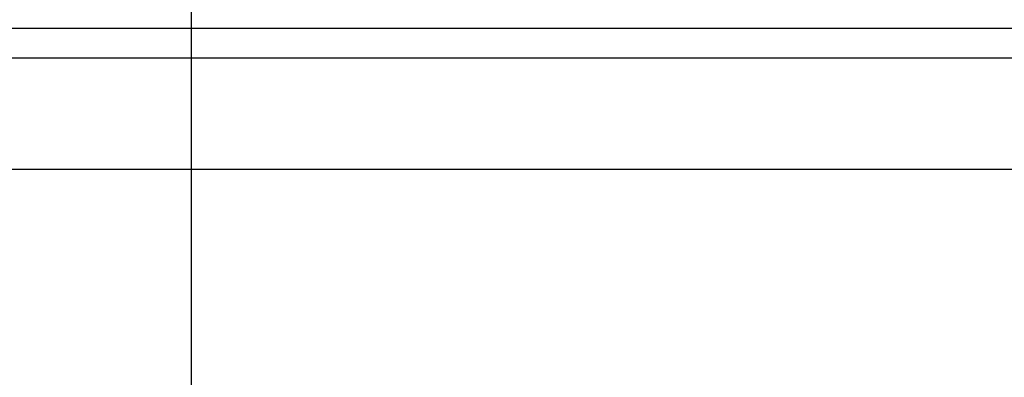
# Model space of a CAD drawing. Units: inches. Extents: x 2278 to 7495, y -71 to 1198.
# Tile 18 of 44: x 5007 to 5060, y 107 to 126. Entities that reach past the tile are written whole.
import ezdxf

# ---------------------------------------------------------------- set-up
doc = ezdxf.new("R2010")
doc.units = ezdxf.units.IN
doc.header["$MEASUREMENT"] = 0
doc.layers.add('A-ANNO-DIMS', color=2, linetype='Continuous', lineweight=18)
doc.layers.add('A-ELEV', color=7, linetype='Continuous', lineweight=25)
doc.styles.get("Standard").update_dxf_attribs({"font": 'arial.ttf'})
doc.dimstyles.get("Standard").update_dxf_attribs({"dimtxt": 6, "dimasz": 3, "dimexe": 0.18, "dimexo": 0.0625, "dimgap": 0.09, "dimtad": 0, "dimtih": 1, "dimtoh": 1, "dimdec": 0, "dimzin": 0, "dimdsep": 46, "dimlunit": 3, "dimtxsty": 'Standard', "dimblk": 'ARCHTICK', "dimcen": 0.09, "dimadec": 0, "dimazin": 0, "dimtfac": 1, "dimtdec": 0, "dimtofl": 0, "dimtmove": 0, "dimatfit": 3, "dimfxl": 1, "dimtolj": 1, "dimtzin": 0, "dimarcsym": 0})

# ---------------------------------------------------------------- blocks, each defined once
blk = doc.blocks.new('_ArchTick')
at = {"color": 0, "linetype": 'ByBlock', "const_width": 0.15}
blk.add_lwpolyline([(-0.5, -0.5), (0.5, 0.5)], dxfattribs=at)
blk = doc.blocks.new('*D59')
at = {"layer": 'A-ANNO-DIMS', "color": 0, "lineweight": -2, "transparency": 16777216}
for p, q in [((5096.589, 159.183), (5101.564, 159.183)), ((5101.384, 159.183), (5101.384, 146.185)), ((5101.384, 126.799), (5101.384, 139.796)), ((5096.589, 126.799), (5101.564, 126.799))]:
    blk.add_line(p, q, dxfattribs=at)
at = {"layer": 'Defpoints', "color": 0, "transparency": 16777216}
for p in [(5096.527, 159.183), (5101.384, 159.183), (5096.527, 126.799)]:
    blk.add_point(p, dxfattribs=at)
at = {"layer": 'A-ANNO-DIMS', "color": 0, "lineweight": -2, "transparency": 16777216, "xscale": 3, "yscale": 3, "zscale": 3}
for p, rotation in [((5101.384, 159.183), 90), ((5101.384, 126.799), 270)]:
    blk.add_blockref('_ArchTick', p, dxfattribs=dict(at, rotation=rotation))
at = {"layer": 'A-ANNO-DIMS', "color": 0, "transparency": 16777216, "insert": (5101.384, 142.991), "char_height": 6, "attachment_point": 5}
blk.add_mtext('\\A1;ORNATE BALUSTER 2\'-8 1/2" TYP.', dxfattribs=at)
blk = doc.blocks.new('*D123')
at = {"layer": 'A-ANNO-DIMS', "color": 0, "lineweight": -2, "transparency": 16777216}
for p, q in [((4736.95, 340.157), (4736.95, -23.427)), ((5145.676, -1.81), (5145.676, -23.427)), ((4736.95, -23.247), (4923.929, -23.247)), ((5145.676, -23.247), (4958.697, -23.247))]:
    blk.add_line(p, q, dxfattribs=at)
at = {"layer": 'Defpoints', "color": 0, "transparency": 16777216}
for p in [(4736.95, 340.219), (5145.676, -1.747), (5145.676, -23.247)]:
    blk.add_point(p, dxfattribs=at)
at = {"layer": 'A-ANNO-DIMS', "color": 0, "lineweight": -2, "transparency": 16777216, "xscale": 3, "yscale": 3, "zscale": 3, "rotation": 180}
blk.add_blockref('_ArchTick', (4736.95, -23.247), dxfattribs=at)
at = {"layer": 'A-ANNO-DIMS', "color": 0, "lineweight": -2, "transparency": 16777216, "xscale": 3, "yscale": 3, "zscale": 3}
blk.add_blockref('_ArchTick', (5145.676, -23.247), dxfattribs=at)
at = {"layer": 'A-ANNO-DIMS', "color": 0, "transparency": 16777216, "insert": (4941.313, -23.247), "char_height": 6, "attachment_point": 5}
blk.add_mtext('\\A1;34\'-0 1/2"', dxfattribs=at)
blk = doc.blocks.new('*D129')
at = {"layer": 'A-ANNO-DIMS', "color": 0, "lineweight": -2, "transparency": 16777216}
for p, q in [((4970.676, 60.779), (4970.676, 361.899)), ((4970.676, 361.719), (4978.373, 361.719)), ((5016.176, 361.719), (5008.479, 361.719)), ((5016.176, 99.315), (5016.176, 361.899))]:
    blk.add_line(p, q, dxfattribs=at)
at = {"layer": 'Defpoints', "color": 0, "transparency": 16777216}
for p in [(5016.176, 361.719), (5016.176, 99.253), (4970.676, 60.717)]:
    blk.add_point(p, dxfattribs=at)
at = {"layer": 'A-ANNO-DIMS', "color": 0, "lineweight": -2, "transparency": 16777216, "xscale": 3, "yscale": 3, "zscale": 3, "rotation": 180}
blk.add_blockref('_ArchTick', (4970.676, 361.719), dxfattribs=at)
at = {"layer": 'A-ANNO-DIMS', "color": 0, "lineweight": -2, "transparency": 16777216, "xscale": 3, "yscale": 3, "zscale": 3}
blk.add_blockref('_ArchTick', (5016.176, 361.719), dxfattribs=at)
at = {"layer": 'A-ANNO-DIMS', "color": 0, "transparency": 16777216, "insert": (4993.426, 361.719), "char_height": 6, "attachment_point": 5}
blk.add_mtext('\\A1;3\'-9 1/2"', dxfattribs=at)
blk = doc.blocks.new('*D130')
at = {"layer": 'A-ANNO-DIMS', "color": 0, "lineweight": -2, "transparency": 16777216}
for p, q in [((5016.176, 99.315), (5016.176, 361.899)), ((5016.176, 361.719), (5048.095, 361.719)), ((5096.176, 361.719), (5064.257, 361.719)), ((5096.176, 99.315), (5096.176, 361.899))]:
    blk.add_line(p, q, dxfattribs=at)
at = {"layer": 'Defpoints', "color": 0, "transparency": 16777216}
for p in [(5096.176, 361.719), (5016.176, 99.253), (5096.176, 99.253)]:
    blk.add_point(p, dxfattribs=at)
at = {"layer": 'A-ANNO-DIMS', "color": 0, "lineweight": -2, "transparency": 16777216, "xscale": 3, "yscale": 3, "zscale": 3, "rotation": 180}
blk.add_blockref('_ArchTick', (5016.176, 361.719), dxfattribs=at)
at = {"layer": 'A-ANNO-DIMS', "color": 0, "lineweight": -2, "transparency": 16777216, "xscale": 3, "yscale": 3, "zscale": 3}
blk.add_blockref('_ArchTick', (5096.176, 361.719), dxfattribs=at)
at = {"layer": 'A-ANNO-DIMS', "color": 0, "transparency": 16777216, "insert": (5056.176, 361.719), "char_height": 6, "attachment_point": 5}
blk.add_mtext('\\A1;6\'-8"', dxfattribs=at)

msp = doc.modelspace()

# ---------------------------------------------------------------- linework, layer by layer
at = {"layer": 'A-ELEV'}
for p, q in [((5065.039, 125.821), (4971.673, 125.821)), ((4874.676, 124.253), (5145.676, 124.253)), ((4874.676, 118.253), (5145.676, 118.253))]:
    msp.add_line(p, q, dxfattribs=at)

# ---------------------------------------------------------------- dimensions: what is measured, and where the dimension line sits
at = {"layer": 'A-ANNO-DIMS'}
for base, p1, p2, picture, middle in [((5016.176, 361.719), (4970.676, 60.717), (5016.176, 99.253), '*D129', (4993.426, 361.719)), ((5096.176, 361.719), (5016.176, 99.253), (5096.176, 99.253), '*D130', (5056.176, 361.719)), ((5145.676, -23.247), (4736.95, 340.219), (5145.676, -1.747), '*D123', (4941.313, -23.247))]:
    dim = msp.add_linear_dim(base=base, p1=p1, p2=p2, dimstyle='Standard', override={"dimdec": 1, "dimlfac": 1, "dimrnd": 0, "dimzin": 1, "dimdsep": 46, "dimlunit": 4, "dimfrac": 2}, dxfattribs=at)
    dim.commit()
    dim.dimension.update_dxf_attribs({"geometry": picture, "text_midpoint": middle})
dim = msp.add_linear_dim(base=(5101.384, 159.183), p1=(5096.527, 126.799), p2=(5096.527, 159.183), angle=90, text='ORNATE BALUSTER <> TYP.', dimstyle='Standard', override={"dimdec": 1, "dimrnd": 0, "dimzin": 1, "dimlunit": 4, "dimfrac": 2}, dxfattribs=at)
dim.commit()
dim.dimension.update_dxf_attribs({"geometry": '*D59', "text_midpoint": (5101.384, 142.991)})

doc.saveas('drawing.dxf')
